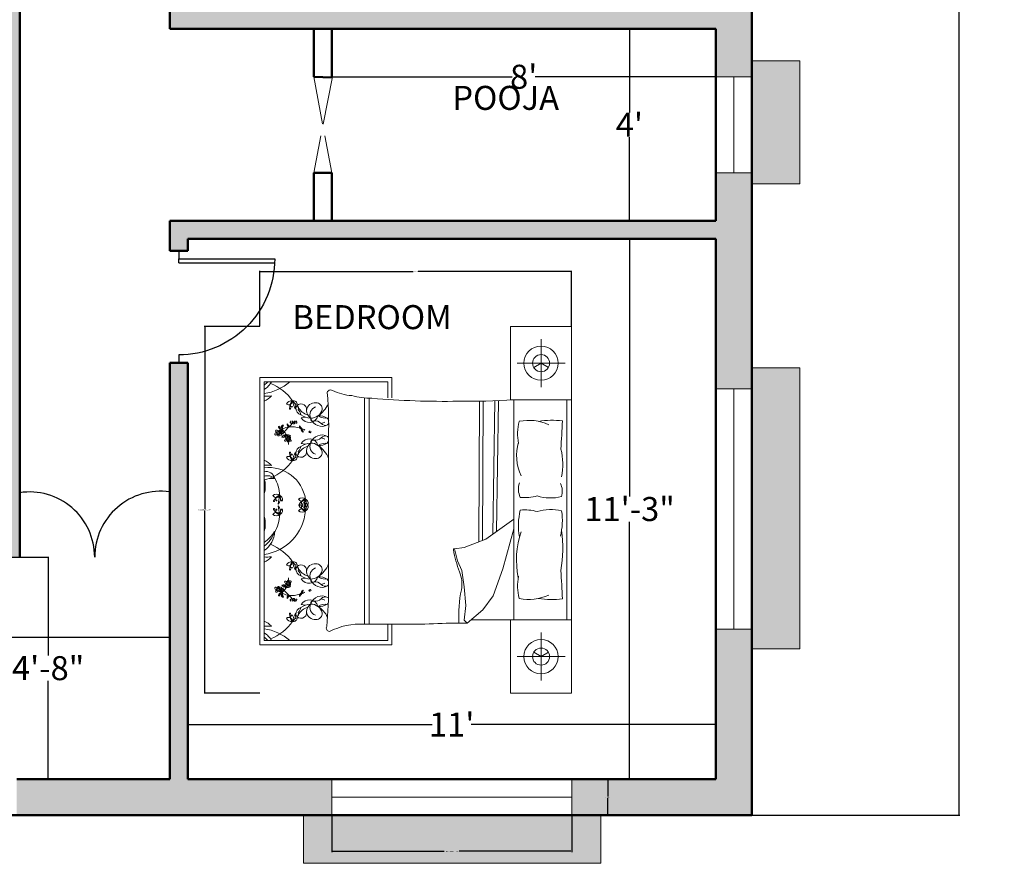
# Model space of a CAD drawing. Units: inches. Extents: x -28 to 544, y -640 to 52.
# Tile 3 of 11: x 297 to 544, y -600 to -389. Entities that reach past the tile are written whole.
import ezdxf

# ---------------------------------------------------------------- set-up
doc = ezdxf.new("R2010")
doc.units = ezdxf.units.IN
doc.header["$MEASUREMENT"] = 0
doc.linetypes.add('ACAD_ISO02W100', pattern=[15, 12, -3])
for name, color, linetype, lineweight in [('A-ANNO-DIMS', 2, 'Continuous', 18), ('A-AREA-IDEN', 7, 'Continuous', 25), ('A-DOOR', 3, 'Continuous', 25), ('A-FLOR-STRS', 7, 'Continuous', 25), ('A-FURN', 8, 'Continuous', 18), ('A-GLAZ', 4, 'Continuous', 20), ('A-ROOF', 8, 'Continuous', 18), ('A-ROOF-PATT', 252, 'Continuous', 13), ('A-WALL', 7, 'Continuous', 50), ('A-WALL-OVHD', 8, 'ACAD_ISO02W100', 18), ('A-WALL-PATT', 5, 'Continuous', 13)]:
    doc.layers.add(name, color=color, linetype=linetype, lineweight=lineweight)
doc.styles.get("Standard").update_dxf_attribs({"font": 'arial.ttf'})
doc.dimstyles.get("Standard").update_dxf_attribs({"dimtxt": 0.18, "dimasz": 0.18, "dimexe": 0.18, "dimexo": 0.0625, "dimgap": 0.09, "dimtad": 0, "dimtih": 1, "dimtoh": 1, "dimdec": 0, "dimzin": 0, "dimdsep": 46, "dimlunit": 3, "dimtxsty": 'Standard', "dimcen": 0.09, "dimadec": 0, "dimazin": 0, "dimtfac": 1, "dimtdec": 0, "dimtofl": 0, "dimtmove": 0, "dimatfit": 3, "dimfxl": 1, "dimtolj": 1, "dimtzin": 0, "dimarcsym": 0})

# ---------------------------------------------------------------- blocks, each defined once
blk = doc.blocks.new('*D23')
at = {"layer": 'A-ANNO-DIMS', "color": 0, "lineweight": -2, "transparency": 16777216}
for p, q in [((339.44, -566.16), (339.44, -564.9)), ((339.62, -565.08), (400.55, -565.08)), ((471.26, -565.08), (410.34, -565.08)), ((471.44, -566.16), (471.44, -564.9))]:
    blk.add_line(p, q, dxfattribs=at)
at = {"layer": 'A-ANNO-DIMS', "color": 0, "transparency": 16777216}
for points in [[(339.62, -565.05), (339.62, -565.11), (339.44, -565.08)], [(471.26, -565.05), (471.26, -565.11), (471.44, -565.08)]]:
    blk.add_solid(points, dxfattribs=at)
at = {"layer": 'Defpoints', "color": 0, "transparency": 16777216}
for p in [(471.44, -565.08), (339.44, -566.22), (471.44, -566.22)]:
    blk.add_point(p, dxfattribs=at)
at = {"layer": 'A-ANNO-DIMS', "color": 0, "transparency": 16777216, "insert": (405.44, -565.08), "char_height": 6, "attachment_point": 5}
blk.add_mtext("\\A1;11'", dxfattribs=at)
blk = doc.blocks.new('*D24')
at = {"layer": 'A-ANNO-DIMS', "color": 0, "lineweight": -2, "transparency": 16777216}
for p, q in [((449.91, -443.92), (449.91, -508.09)), ((449.97, -443.74), (450.09, -443.74)), ((449.91, -578.56), (449.91, -514.4)), ((449.97, -578.74), (450.09, -578.74))]:
    blk.add_line(p, q, dxfattribs=at)
at = {"layer": 'A-ANNO-DIMS', "color": 0, "transparency": 16777216}
for points in [[(449.88, -443.92), (449.94, -443.92), (449.91, -443.74)], [(449.88, -578.56), (449.94, -578.56), (449.91, -578.74)]]:
    blk.add_solid(points, dxfattribs=at)
at = {"layer": 'Defpoints', "color": 0, "transparency": 16777216}
for p in [(449.91, -443.74), (449.91, -578.74), (449.91, -578.74)]:
    blk.add_point(p, dxfattribs=at)
at = {"layer": 'A-ANNO-DIMS', "color": 0, "transparency": 16777216, "insert": (449.91, -511.24), "char_height": 6, "attachment_point": 5}
blk.add_mtext('\\A1;11\'-3"', dxfattribs=at)
blk = doc.blocks.new('*D28')
at = {"layer": 'A-ANNO-DIMS', "color": 0, "lineweight": -2, "transparency": 16777216}
for p, q in [((480.51, 7.76), (532.47, 7.76)), ((532.29, 7.58), (532.29, -286.84)), ((532.29, -587.56), (532.29, -293.14)), ((480.51, -587.74), (532.47, -587.74))]:
    blk.add_line(p, q, dxfattribs=at)
at = {"layer": 'A-ANNO-DIMS', "color": 0, "transparency": 16777216}
for points in [[(532.26, 7.58), (532.32, 7.58), (532.29, 7.76)], [(532.26, -587.56), (532.32, -587.56), (532.29, -587.74)]]:
    blk.add_solid(points, dxfattribs=at)
at = {"layer": 'Defpoints', "color": 0, "transparency": 16777216}
for p in [(480.44, 7.76), (480.44, -587.74), (532.29, -587.74)]:
    blk.add_point(p, dxfattribs=at)
at = {"layer": 'A-ANNO-DIMS', "color": 0, "transparency": 16777216, "insert": (532.29, -289.99), "char_height": 6, "attachment_point": 5}
blk.add_mtext('\\A1;49\'-8"', dxfattribs=at)
blk = doc.blocks.new('*D31')
at = {"layer": 'A-ANNO-DIMS', "color": 0, "lineweight": -2, "transparency": 16777216}
for p, q in [((375.44, -397.6), (375.44, -403.42)), ((471.44, -397.6), (471.44, -403.42)), ((375.62, -403.24), (420.59, -403.24)), ((471.26, -403.24), (426.3, -403.24))]:
    blk.add_line(p, q, dxfattribs=at)
at = {"layer": 'A-ANNO-DIMS', "color": 0, "transparency": 16777216}
for points in [[(375.62, -403.21), (375.62, -403.27), (375.44, -403.24)], [(471.26, -403.21), (471.26, -403.27), (471.44, -403.24)]]:
    blk.add_solid(points, dxfattribs=at)
at = {"layer": 'Defpoints', "color": 0, "transparency": 16777216}
for p in [(375.44, -397.54), (471.44, -397.54), (471.44, -403.24)]:
    blk.add_point(p, dxfattribs=at)
at = {"layer": 'A-ANNO-DIMS', "color": 0, "transparency": 16777216, "insert": (423.44, -403.24), "char_height": 6, "attachment_point": 5}
blk.add_mtext("\\A1;8'", dxfattribs=at)
blk = doc.blocks.new('*D32')
at = {"layer": 'A-ANNO-DIMS', "color": 0, "lineweight": -2, "transparency": 16777216}
for p, q in [((453.92, -391.24), (449.68, -391.24)), ((449.86, -391.42), (449.86, -412.15)), ((449.86, -439.06), (449.86, -418.33)), ((453.92, -439.24), (449.68, -439.24))]:
    blk.add_line(p, q, dxfattribs=at)
at = {"layer": 'A-ANNO-DIMS', "color": 0, "transparency": 16777216}
for points in [[(449.83, -391.42), (449.89, -391.42), (449.86, -391.24)], [(449.83, -439.06), (449.89, -439.06), (449.86, -439.24)]]:
    blk.add_solid(points, dxfattribs=at)
at = {"layer": 'Defpoints', "color": 0, "transparency": 16777216}
for p in [(453.98, -391.24), (449.86, -439.24), (453.98, -439.24)]:
    blk.add_point(p, dxfattribs=at)
at = {"layer": 'A-ANNO-DIMS', "color": 0, "transparency": 16777216, "insert": (449.86, -415.24), "char_height": 6, "attachment_point": 5}
blk.add_mtext("\\A1;4'", dxfattribs=at)
blk = doc.blocks.new('*D41')
at = {"layer": 'A-ANNO-DIMS', "color": 0, "lineweight": -2, "transparency": 16777216}
for p, q in [((162.44, -543.27), (162.44, -543.15)), ((162.62, -543.33), (238.58, -543.33)), ((334.76, -543.33), (258.81, -543.33)), ((334.94, -543.27), (334.94, -543.15))]:
    blk.add_line(p, q, dxfattribs=at)
at = {"layer": 'A-ANNO-DIMS', "color": 0, "transparency": 16777216}
for points in [[(162.62, -543.3), (162.62, -543.36), (162.44, -543.33)], [(334.76, -543.3), (334.76, -543.36), (334.94, -543.33)]]:
    blk.add_solid(points, dxfattribs=at)
at = {"layer": 'Defpoints', "color": 0, "transparency": 16777216}
for p in [(162.44, -543.33), (334.94, -543.33), (334.94, -543.33)]:
    blk.add_point(p, dxfattribs=at)
at = {"layer": 'A-ANNO-DIMS', "color": 0, "transparency": 16777216, "insert": (248.69, -543.33), "char_height": 6, "attachment_point": 5}
blk.add_mtext('\\A1;14\'-5"', dxfattribs=at)
blk = doc.blocks.new('*D42')
at = {"layer": 'A-ANNO-DIMS', "color": 0, "lineweight": -2, "transparency": 16777216}
for p, q in [((297.51, -523.24), (304.73, -523.24)), ((304.55, -523.42), (304.55, -547.84)), ((304.55, -578.56), (304.55, -554.14)), ((301.15, -578.74), (304.73, -578.74))]:
    blk.add_line(p, q, dxfattribs=at)
at = {"layer": 'A-ANNO-DIMS', "color": 0, "transparency": 16777216}
for points in [[(304.52, -523.42), (304.58, -523.42), (304.55, -523.24)], [(304.52, -578.56), (304.58, -578.56), (304.55, -578.74)]]:
    blk.add_solid(points, dxfattribs=at)
at = {"layer": 'Defpoints', "color": 0, "transparency": 16777216}
for p in [(297.44, -523.24), (301.09, -578.74), (304.55, -578.74)]:
    blk.add_point(p, dxfattribs=at)
at = {"layer": 'A-ANNO-DIMS', "color": 0, "transparency": 16777216, "insert": (304.55, -550.99), "char_height": 6, "attachment_point": 5}
blk.add_mtext('\\A1;4\'-8"', dxfattribs=at)
blk = doc.blocks.new('BED-DOUBLE-HEADBOARD-92')
for p, q in [((77.93, 0), (77.93, 91.63)), ((70.29, 76.48), (70.29, 88.45)), ((64.3, 82.47), (76.28, 82.47)), ((0, 78.9), (0, 12.09)), ((33.01, 78.9), (0, 78.9)), ((33.01, 73.82), (33.01, 78.9)), ((1.06, 77.84), (31.95, 77.84)), ((1.06, 13.16), (1.06, 77.84)), ((31.95, 77.84), (31.95, 73.8)), ((26.15, 73.81), (26.15, 17.27)), ((27.29, 73.72), (27.29, 17.27)), ((54.87, 72.98), (54.73, 37.82)), ((55.81, 72.98), (55.68, 38.18)), ((58.7, 73.02), (58.23, 39.75)), ((59.64, 73.06), (59.18, 40.44)), ((63.45, 18.33), (63.45, 73.3)), ((76.75, 73.3), (76.75, 18.33)), ((10.35, 68.81), (11.39, 69.01)), ((17.15, 64.42), (17.15, 27.21)), ((10.35, 62.4), (11.39, 62.2)), ((63.45, 43.5), (56.46, 38.48)), ((60.72, 31.05), (63.45, 41.05)), ((56.46, 38.48), (51.08, 36.44)), ((51.08, 36.44), (48.67, 36.07)), ((48.67, 36.07), (49.41, 33.1)), ((49.41, 33.1), (50.52, 30.68)), ((50.52, 30.68), (51.08, 26.6)), ((58.31, 24.37), (60.72, 31.05)), ((10.35, 28.59), (11.39, 28.79)), ((51.08, 26.6), (51.45, 21.96)), ((10.35, 22.19), (11.39, 21.98)), ((55.71, 20.85), (58.31, 24.37)), ((51.45, 21.96), (51.08, 18.25)), ((51.82, 17.51), (55.71, 20.85)), ((31.95, 17.28), (31.95, 13.16)), ((33.01, 12.09), (33.01, 17.28)), ((51.08, 18.25), (51.82, 17.51)), ((77.93, 18.33), (52.78, 18.33)), ((70.29, 15.15), (70.29, 3.18)), ((31.95, 13.16), (1.06, 13.16)), ((0, 12.09), (33.01, 12.09)), ((64.3, 9.16), (76.28, 9.16))]:
    blk.add_line(p, q)
for points in [[(77.93, 73.3), (62.65, 73.3), (62.65, 91.63), (77.93, 91.63)], [(70.29, 82.47), (68.44, 81.4)], [(70.29, 82.47), (72.14, 81.4)], [(62.65, 18.33), (62.65, 0), (77.93, 0)], [(70.29, 9.16), (68.44, 10.23)], [(70.29, 9.16), (72.14, 10.23)]]:
    blk.add_lwpolyline(points)
for points in [[(28.01, 73.7, -0.056112), (22.97, 74.36, -0.095341), (18.12, 75.65)], [(75.64, 68.04, 0.074897), (69.66, 67.93, -0.472817)], [(69.32, 49.3, 0.14099), (75.43, 49.12, 0.235245)], [(69.32, 45.39, -0.14099), (75.43, 45.57, -0.235245)], [(75.64, 23.59, -0.074897), (69.66, 23.7, 0.472817)], [(43.43, 17.31, -0.001242), (26.04, 17.27, 0.127202), (17.38, 15.43)]]:
    blk.add_lwpolyline(points, format="xyb")
for centre, radius in [((70.29, 82.47), 4.28), ((70.29, 82.47), 2.14), ((4.57, 65.04), 0.233), ((7.03, 63.51), 0.233), ((7.03, 27.48), 0.233), ((4.57, 25.95), 0.233), ((70.29, 9.16), 4.28), ((70.29, 9.16), 2.14)]:
    blk.add_circle(centre, radius)
for centre, radius, start, end in [((-2.15, 80.74), 5.83, 303.4617, 330.1116), ((-3.24, 82.84), 7.27, 306.3036, 316.4814), ((-0.55, 86.74), 11.97, 277.745, 311.8856), ((-1.73, 66.27), 11.97, 34.3865, 68.5908), ((-0.8, 77.48), 4.87, 292.5547, 318.9546), ((1.81, 90.8), 16.56, 267.4081, 273.6519), ((17.65, 74.95), 0.835, 56.1736, 203.4781), ((-71.97, 67.22), 89.16, 358.1965, 4.7598), ((7.86, 71.73), 1.33, 77.7115, 159.0387), ((7.14, 73.06), 0.999, 238.4633, 358.2869), ((10.42, 71.04), 3.03, 138.8402, 177.9352), ((8.6, 72.16), 0.979, 117.6827, 223.7762), ((8.03, 71.59), 0.078, 223.7729, 159.7333), ((8.38, 72.07), 0.992, 2.9516, 103.728), ((16.31, 74.84), 8.37, 192.5173, 207.1824), ((7.04, 71.5), 1.89, 345.4653, 54.2343), ((9.89, 74.09), 2.04, 211.3827, 255.2969), ((10.28, 70.9), 1.38, 350.264, 160.8688), ((8.79, 71.18), 0.843, 333.9755, 53.2681), ((13.81, 70.4), 2.19, 84.9449, 172.8857), ((14.64, 69.54), 2.13, 111.5819, 201.4221), ((14.03, 71.03), 1.55, 354.4856, 91.0538), ((10.7, 75.07), 6.94, 303.6671, 336.3547), ((46.26, 287.69), 214.77, 265.1265, 270.8855), ((52.25, 237.57), 164.64, 269.0718, 273.9), ((7.54, 71.14), 0.149, 177.9352, 11.4834), ((7.62, 71.16), 0.0722, 11.4834, 127.9409), ((10.69, 71.23), 1.72, 175.969, 254.3045), ((8.41, 69.38), 1.83, 6.1662, 51.5825), ((13.3, 73.63), 4.33, 211.2614, 251.7045), ((12.96, 73.67), 4.92, 236.2883, 266.5076), ((12.33, 69.94), 2.28, 209.9085, 343.1337), ((14.29, 70.78), 2.66, 182.3591, 234.0401), ((12.88, 71.51), 2.76, 265.2933, 346.921), ((16.47, 72.53), 3.8, 238.8218, 280.751), ((14.82, 65.78), 3.53, 55.785, 94.7304), ((4.91, 66.54), 0.261, 124.3538, 214.3923), ((5.47, 66.72), 0.705, 176.9701, 248.2913), ((10.5, 70.44), 6.82, 212.6784, 216.3746), ((5.88, 66.37), 0.608, 122.8155, 187.3992), ((6.14, 66.29), 0.705, 109.4799, 177.6828), ((5.76, 66.74), 0.261, 56.8636, 146.9021), ((5.9, 66.45), 0.27, 148.8844, 224.2646), ((11.5, 63.06), 6.82, 145.1882, 148.8844), ((7.62, 62.77), 3.8, 94.756, 119.2041), ((15.72, 57.29), 12.52, 132.2412, 142.1744), ((9.4, 67.26), 2.58, 178.3264, 187.1302), ((6.61, 66.9), 0.481, 11.3256, 64.4621), ((8.24, 67.59), 1.45, 190.2588, 210.656), ((7.27, 67), 0.44, 188.3432, 274.2869), ((7.66, 67.24), 0.768, 210.656, 242.6341), ((8.24, 67.9), 1.47, 218.2101, 226.3071), ((7.15, 66.67), 0.187, 325.7657, 67.4417), ((1.35, 72.91), 8.7, 313.1541, 322.0459), ((7.81, 58.99), 7.59, 73.5842, 93.8277), ((7.75, 67.68), 0.179, 142.4737, 265.053), ((7.99, 67.72), 0.385, 127.7621, 169.0403), ((7.78, 68.04), 0.542, 265.053, 338.3618), ((8.5, 67.3), 0.709, 113.4276, 137.6104), ((8.42, 68.04), 0.233, 183.2768, 356.7232), ((8.59, 67.61), 0.382, 139.7889, 227.6792), ((8.47, 67.48), 0.201, 227.6792, 350.3487), ((7.69, 67.62), 0.764, 353.0852, 15.7171), ((8.19, 67.53), 0.482, 350.3487, 43.6538), ((9.08, 68.03), 0.561, 198.7263, 262.5032), ((8.64, 67.76), 0.223, 1.1081, 91.8675), ((9.06, 67.64), 0.18, 255.2356, 54.9248), ((8.78, 67.71), 0.389, 11.5637, 52.6358), ((12.48, 66.71), 2.58, 178.3264, 187.1302), ((9.69, 66.35), 0.481, 11.3256, 64.4621), ((11.32, 67.04), 1.45, 190.2588, 210.656), ((13.28, 68.5), 0.569, 167.3041, 285.1471), ((14.82, 65.78), 3.53, 122.7011, 126.3445), ((15.49, 69.59), 2.92, 199.2822, 299.1751), ((13.92, 66.14), 1.88, 41.5653, 105.1471), ((14.96, 70.03), 2.63, 277.436, 299.9149), ((16.35, 68.29), 1.37, 221.5653, 293.8354), ((16.14, 67.83), 1.1, 17.4186, 52.325), ((16.14, 67.83), 1.1, 314.4517, 343.3657), ((76.71, 64.77), 12.28, 165.1039, 191.0369), ((67.25, 56.37), 11.81, 65.1316, 101.7583), ((947.66, 17.54), 873.48, 176.68521, 177.14978), ((3.9, 64.68), 0.179, 142.4737, 265.053), ((4.14, 64.72), 0.385, 61.2196, 169.0403), ((3.93, 65.05), 0.542, 265.053, 338.3618), ((4.39, 65.51), 0.461, 157.4086, 261.4386), ((4.13, 65.53), 0.231, 58.0499, 135.6268), ((4.65, 64.3), 0.709, 113.4276, 137.6104), ((4.37, 65.38), 0.155, 172.906, 277.132), ((3.87, 65.1), 0.736, 14.7558, 58.0499), ((4.74, 64.62), 0.382, 139.7889, 227.6792), ((4.62, 64.48), 0.201, 227.6792, 350.3487), ((4.9, 65.3), 0.318, 36.1046, 181.4281), ((3.84, 64.62), 0.764, 353.0852, 15.7171), ((4.34, 64.53), 0.482, 350.3487, 43.6538), ((5.29, 66.5), 0.608, 190.3057, 287.1958), ((4.71, 65.55), 0.321, 270.0645, 331.1507), ((4.98, 65.47), 0.367, 221.8413, 265.7877), ((5.24, 65.03), 0.561, 198.7263, 262.5032), ((4.79, 64.77), 0.223, 1.1081, 91.8675), ((4.98, 65.33), 0.229, 263.7526, 41.7054), ((4.93, 64.72), 0.389, 11.5637, 86.365), ((5.23, 66.56), 0.27, 216.3746, 291.7548), ((7.62, 62.77), 3.8, 124.0033, 132.4917), ((5.21, 64.65), 0.18, 255.2356, 54.9248), ((3.7, 62.29), 4.06, 63.7819, 68.2913), ((5.88, 65.42), 0.647, 128.3208, 208.8162), ((5.99, 65.47), 0.773, 207.7043, 254.3516), ((5.41, 66.12), 0.204, 289.3605, 111.7548), ((5.56, 66.12), 0.204, 221.8703, 44.2646), ((6.48, 65.52), 1.06, 157.2305, 229.0635), ((5.49, 65.02), 1.06, 270.278, 342.111), ((6.2, 63.69), 0.752, 98.7227, 159.3375), ((6.12, 65.88), 0.626, 174.4544, 220.6188), ((2.56, 62.38), 4.56, 30.544, 49.818), ((5.08, 64.98), 0.752, 340.0041, 40.6188), ((5.99, 65.06), 0.626, 278.7227, 324.8872), ((5.88, 64.55), 0.647, 290.5253, 358.5375), ((6.85, 63.99), 0.461, 157.4086, 261.4386), ((6.59, 64), 0.231, 58.0499, 135.6268), ((7.14, 64.73), 0.647, 182.8499, 266.1226), ((6.89, 65.19), 0.626, 231.7607, 277.9252), ((7.38, 65.3), 1.06, 214.5369, 286.3699), ((6.33, 63.57), 0.736, 14.7558, 58.0499), ((2.56, 62.38), 4.56, 23.0501, 23.8477), ((7.08, 63.82), 0.752, 37.3105, 97.9252), ((7.36, 63.77), 0.318, 36.1046, 181.4281), ((7.16, 64.86), 0.773, 265.0106, 311.658), ((10.35, 66.45), 0.44, 188.3432, 274.2869), ((10.74, 66.7), 0.768, 210.656, 242.6341), ((11.32, 67.36), 1.47, 218.2101, 226.3071), ((10.23, 66.12), 0.187, 325.7657, 67.4417), ((10.76, 65.78), 0.44, 147.5332, 233.4768), ((11.15, 66), 0.768, 179.1859, 211.164), ((10.41, 65.83), 0.187, 354.3784, 96.0543), ((7.81, 58.99), 7.59, 63.0032, 69.8941), ((11.99, 67.54), 2.58, 234.6898, 243.4936), ((11.74, 66.36), 1.45, 211.164, 231.5612), ((12.01, 66.21), 1.47, 195.5129, 203.6099), ((10.35, 65.24), 0.481, 357.3579, 50.4944), ((12.42, 65.34), 0.177, 12.7051, 190.4384), ((12.53, 65.36), 0.287, 190.4384, 10.4136), ((15.49, 61.62), 2.92, 60.8249, 160.7178), ((16.35, 62.91), 1.37, 66.1646, 138.4347), ((16.14, 63.38), 1.1, 23.2856, 45.5483), ((5.82, 64.66), 0.773, 244.9899, 291.6373), ((6.36, 63.16), 0.179, 142.4737, 265.053), ((6.6, 63.19), 0.385, 61.2196, 169.0403), ((6.39, 63.52), 0.542, 265.053, 338.3618), ((7.11, 62.78), 0.709, 113.4276, 137.6104), ((6.83, 63.86), 0.155, 172.906, 277.132), ((7.2, 63.09), 0.382, 139.7889, 227.6792), ((7.08, 62.96), 0.201, 227.6792, 350.3487), ((6.3, 63.09), 0.764, 353.0852, 15.7171), ((2.56, 62.38), 4.56, 357.1071, 4.7585), ((6.8, 63), 0.482, 350.3487, 43.6538), ((7.17, 64.02), 0.321, 270.0645, 331.1507), ((7.44, 63.94), 0.367, 221.8413, 265.7877), ((7.7, 63.5), 0.561, 198.7263, 262.5032), ((7.25, 63.24), 0.223, 1.1081, 91.8675), ((7.44, 63.81), 0.229, 263.7526, 41.7054), ((7.39, 63.19), 0.389, 11.5637, 86.365), ((7.67, 63.12), 0.18, 255.2356, 54.9248), ((10.69, 59.98), 1.72, 105.6955, 184.031), ((8.41, 61.83), 1.83, 308.4175, 353.8338), ((13.3, 57.58), 4.33, 108.2955, 148.7386), ((12.96, 57.54), 4.92, 93.4924, 123.7117), ((12.33, 61.27), 2.28, 16.8663, 150.0915), ((14.29, 60.43), 2.66, 125.9599, 177.6409), ((14.64, 61.67), 2.13, 158.5779, 248.4181), ((12.88, 59.7), 2.76, 13.079, 94.7067), ((13.28, 62.71), 0.569, 74.8529, 192.6959), ((14.82, 65.43), 3.53, 233.6555, 237.2989), ((13.92, 65.07), 1.88, 254.8529, 318.4347), ((16.47, 58.68), 3.8, 79.7133, 121.1782), ((14.82, 65.43), 3.53, 265.2696, 304.215), ((10.7, 56.14), 6.94, 21.4941, 56.3329), ((14.96, 61.18), 2.63, 60.0851, 82.564), ((16.14, 63.38), 1.1, 307.675, 336.7144), ((75.81, 59.47), 11.66, 163.8254, 206.1239), ((7.14, 58.15), 0.999, 1.7131, 121.5367), ((7.54, 60.07), 0.149, 348.5166, 182.0648), ((10.42, 60.17), 3.03, 182.0648, 221.1598), ((7.62, 60.05), 0.0722, 232.0591, 348.5166), ((8.6, 59.04), 0.979, 136.2238, 242.3173), ((7.98, 59.63), 0.129, 200.2817, 136.2238), ((7.04, 59.71), 1.89, 305.7657, 14.5347), ((16.31, 56.36), 8.37, 152.8176, 167.4827), ((8.38, 59.14), 0.992, 256.272, 357.0484), ((9.89, 57.11), 2.04, 104.7031, 148.6173), ((10.28, 60.31), 1.38, 199.1312, 9.736), ((8.79, 60.02), 0.843, 306.7319, 26.0245), ((13.81, 60.81), 2.19, 187.1143, 275.0551), ((14.03, 60.18), 1.55, 268.9462, 5.5144), ((59.61, 57.17), 16.11, 348.8159, 13.6573), ((-0.8, 53.73), 4.87, 41.0454, 67.4453), ((1.81, 40.41), 16.56, 86.3481, 92.5919), ((-1.73, 64.94), 11.97, 291.4092, 325.6135), ((7.86, 59.47), 1.33, 200.9613, 282.2885), ((2.21, 47.13), 9.26, 8.1803, 97.1364), ((1.57, 53.24), 2.15, 10.9261, 103.6102), ((1.86, 51.63), 2.72, 48.0951, 107.1391), ((-5.23, 51.78), 6.58, 343.5431, 17.0202), ((3.06, 48.33), 5.36, 83.3805, 111.883), ((-6.96, 48.43), 11.97, 4.4623, 27.4146), ((69.49, 50.99), 4.86, 161.4593, 204.9817), ((71.07, 50.37), 4.53, 343.8974, 26.6563), ((-8.62, 49.17), 9.73, 4.3787, 5.6357), ((-15.29, 44.05), 17.39, 19.7217, 19.9028), ((4.08, 48.38), 1.33, 47.7873, 129.1145), ((4.12, 49.89), 0.999, 208.5391, 328.3627), ((5.95, 46.5), 3.03, 108.9159, 148.011), ((4.93, 48.39), 0.979, 87.7585, 193.852), ((12.96, 46.86), 8.37, 162.593, 177.2582), ((3.25, 48.59), 1.89, 315.5411, 24.3101), ((7.01, 49.42), 2.04, 181.4585, 225.3727), ((4.69, 48.41), 0.992, 333.0274, 73.8037), ((66.26, 60.1), 11.23, 264.0129, 285.8293), ((3.51, 48.03), 0.149, 148.011, 341.5592), ((3.58, 48), 0.0722, 341.5592, 98.0167), ((4.16, 48.17), 0.078, 193.9791, 129.8091), ((12.96, 47.19), 8.37, 182.7418, 197.407), ((3.25, 45.46), 1.89, 335.6899, 44.4589), ((10.49, 47.47), 1.33, 47.7873, 129.1145), ((10.53, 48.97), 0.999, 208.5391, 328.3627), ((9.92, 47.11), 0.149, 148.011, 341.5592), ((9.92, 46.94), 0.149, 18.4408, 211.989), ((12.36, 45.59), 3.03, 108.9159, 148.011), ((12.36, 48.46), 3.03, 211.989, 251.0841), ((9.99, 47.09), 0.0722, 341.5592, 98.0167), ((9.99, 46.96), 0.0722, 261.9833, 18.4408), ((11.34, 47.47), 0.979, 87.7585, 193.852), ((11.34, 46.58), 0.979, 166.148, 272.2415), ((10.52, 46.78), 0.129, 230.0755, 166.148), ((10.57, 47.26), 0.078, 193.9791, 129.8091), ((9.65, 47.67), 1.89, 315.5411, 24.3101), ((19.37, 45.95), 8.37, 162.593, 177.2582), ((9.65, 46.38), 1.89, 335.6899, 44.4589), ((19.37, 48.1), 8.37, 182.7418, 197.407), ((11.1, 47.5), 0.992, 333.0274, 73.8037), ((13.42, 48.5), 2.04, 181.4585, 225.3727), ((11.1, 46.55), 0.992, 286.1963, 26.9726), ((13.42, 45.55), 2.04, 134.6273, 178.5415), ((-0.55, 46.53), 11.97, 277.745, 355.5377), ((4.12, 44.16), 0.999, 31.6373, 151.4609), ((4.08, 45.66), 1.33, 230.8855, 312.2127), ((3.51, 46.02), 0.149, 18.4408, 211.989), ((5.95, 47.54), 3.03, 211.989, 251.0841), ((3.58, 46.04), 0.0722, 261.9833, 18.4408), ((-6.96, 45.61), 11.97, 332.5854, 355.5377), ((4.93, 45.66), 0.979, 166.148, 272.2415), ((4.11, 45.86), 0.129, 230.0755, 166.148), ((7.01, 44.63), 2.04, 134.6273, 178.5415), ((4.69, 45.63), 0.992, 286.1963, 26.9726), ((10.53, 45.07), 0.999, 31.6373, 151.4609), ((10.49, 46.58), 1.33, 230.8855, 312.2127), ((80.79, 41.94), 16.16, 166.3762, 190.1383), ((66.26, 34.58), 11.23, 74.1707, 95.9871), ((59.28, 43.16), 16.33, 346.04, 8.4751), ((-5.23, 42.27), 6.58, 342.9798, 16.4569), ((-8.62, 44.87), 9.73, 354.3643, 355.6213), ((-15.29, 50), 17.39, 340.0972, 340.2783), ((-2.15, 40.53), 5.83, 303.4617, 358.728), ((-5.28, 46.44), 10.81, 305.947, 325.9877), ((-3.24, 42.62), 7.27, 306.3036, 342.1496), ((85.44, 33.32), 21.3, 160.7385, 191.9603), ((42.48, 36.14), 33.23, 350.503, 7.7804), ((-1.73, 26.06), 11.97, 34.3865, 68.5908), ((48.59, 35.86), 0.221, 70.2464, 181.1377), ((83.29, 42.43), 35.54, 190.6617, 199.8806), ((1.81, 50.59), 16.56, 267.4081, 273.6519), ((-0.8, 37.26), 4.87, 292.5547, 318.9546), ((7.86, 31.52), 1.33, 77.7115, 159.0387), ((7.14, 32.84), 0.999, 238.4633, 358.2869), ((10.42, 30.82), 3.03, 138.8402, 177.9352), ((8.6, 31.95), 0.979, 117.6827, 223.7762), ((8.38, 31.85), 0.992, 2.9516, 103.728), ((9.89, 33.88), 2.04, 211.3827, 255.2969), ((7.04, 31.28), 1.89, 345.4653, 54.2343), ((16.31, 34.63), 8.37, 192.5173, 207.1824), ((10.28, 30.69), 1.38, 350.264, 160.8688), ((13.81, 30.18), 2.19, 84.9449, 172.8857), ((14.03, 30.82), 1.55, 354.4856, 91.0538), ((10.7, 34.86), 6.94, 303.6671, 338.5059), ((7.54, 30.93), 0.149, 177.9352, 11.4834), ((7.62, 30.94), 0.0722, 11.4834, 127.9409), ((8.03, 31.37), 0.078, 223.7729, 159.7333), ((10.69, 31.02), 1.72, 175.969, 254.3045), ((8.79, 30.97), 0.843, 333.9755, 53.2681), ((8.41, 29.17), 1.83, 6.1662, 51.5825), ((13.3, 33.41), 4.33, 211.2614, 251.7045), ((14.29, 30.56), 2.66, 182.3591, 234.0401), ((14.64, 29.32), 2.13, 111.5819, 201.4221), ((12.88, 31.29), 2.76, 265.2933, 346.921), ((43.05, 27.34), 7.46, 348.6608, 23.7384), ((947.66, 74.1), 873.48, 182.85022, 183.31479), ((5.82, 26.33), 0.773, 68.3627, 115.0101), ((6.36, 27.83), 0.179, 94.947, 217.5263), ((6.6, 27.8), 0.385, 190.9597, 298.7804), ((6.39, 27.47), 0.542, 21.6382, 94.947), ((6.85, 27), 0.461, 98.5614, 202.5914), ((7.11, 28.21), 0.709, 222.3896, 246.5724), ((6.83, 27.13), 0.155, 82.868, 187.094), ((6.33, 27.42), 0.736, 301.9501, 345.2442), ((7.2, 27.9), 0.382, 132.3208, 220.2111), ((7.08, 28.04), 0.201, 9.6513, 132.3208), ((6.3, 27.9), 0.764, 344.2829, 6.9148), ((7.36, 27.22), 0.318, 178.5719, 323.8954), ((2.56, 28.61), 4.56, 355.2415, 2.8929), ((6.8, 27.99), 0.482, 316.3462, 9.6513), ((7.7, 27.49), 0.561, 97.4968, 161.2737), ((7.44, 27.05), 0.367, 94.2123, 138.1587), ((7.17, 26.97), 0.321, 28.8493, 89.9355), ((7.25, 27.75), 0.223, 268.1325, 358.8919), ((7.39, 27.8), 0.389, 273.635, 348.4363), ((7.44, 27.19), 0.229, 318.2946, 96.2474), ((7.67, 27.87), 0.18, 305.0752, 104.7644), ((12.96, 33.45), 4.92, 236.2883, 266.5076), ((12.33, 29.73), 2.28, 209.9085, 343.1337), ((13.28, 28.28), 0.569, 167.3041, 285.1471), ((14.82, 25.56), 3.53, 122.7011, 126.3445), ((15.49, 29.37), 2.92, 199.2822, 299.1751), ((13.92, 25.92), 1.88, 41.5653, 105.1471), ((16.47, 32.31), 3.8, 238.8218, 280.2867), ((14.82, 25.56), 3.53, 55.785, 94.7304), ((14.96, 29.81), 2.63, 277.436, 299.9149), ((16.35, 28.08), 1.37, 221.5653, 293.8354), ((-78.23, 26.12), 95.39, 354.3113, 0.6567), ((16.14, 27.61), 1.1, 23.2856, 52.325), ((16.14, 27.61), 1.1, 314.4517, 336.771), ((76.71, 26.86), 12.28, 168.9631, 194.8961), ((3.9, 26.31), 0.179, 94.947, 217.5263), ((4.14, 26.27), 0.385, 190.9597, 298.7804), ((3.93, 25.95), 0.542, 21.6382, 94.947), ((4.39, 25.48), 0.461, 98.5614, 202.5914), ((4.13, 25.46), 0.231, 224.3732, 301.9501), ((4.65, 26.69), 0.709, 222.3896, 246.5724), ((4.37, 25.61), 0.155, 82.868, 187.094), ((3.87, 25.89), 0.736, 301.9501, 345.2442), ((4.74, 26.38), 0.382, 132.3208, 220.2111), ((4.62, 26.51), 0.201, 9.6513, 132.3208), ((3.84, 26.37), 0.764, 344.2829, 6.9148), ((4.9, 25.7), 0.318, 178.5719, 323.8954), ((4.34, 26.46), 0.482, 316.3462, 9.6513), ((5.29, 24.49), 0.608, 72.8042, 169.6943), ((5.24, 25.96), 0.561, 97.4968, 161.2737), ((4.98, 25.52), 0.367, 94.2123, 138.1587), ((4.71, 25.45), 0.321, 28.8493, 89.9355), ((5.47, 24.27), 0.705, 111.7087, 183.0299), ((4.79, 26.23), 0.223, 268.1325, 358.8919), ((4.93, 26.28), 0.389, 273.635, 348.4363), ((4.98, 25.66), 0.229, 318.2946, 96.2474), ((5.23, 24.44), 0.27, 68.2452, 143.6254), ((7.62, 28.22), 3.8, 227.5083, 235.9967), ((5.21, 26.35), 0.18, 305.0752, 104.7644), ((3.7, 28.7), 4.06, 291.7087, 296.2181), ((5.88, 25.57), 0.647, 151.1838, 231.6792), ((5.88, 24.62), 0.608, 172.6008, 237.1845), ((5.99, 25.53), 0.773, 105.6484, 152.2957), ((5.41, 24.88), 0.204, 248.2452, 70.6395), ((5.56, 24.88), 0.204, 315.7354, 138.1297), ((6.48, 25.47), 1.06, 130.9365, 202.7695), ((6.14, 24.7), 0.705, 182.3172, 250.5201), ((5.49, 25.97), 1.06, 17.889, 89.722), ((6.2, 27.3), 0.752, 200.6625, 261.2773), ((6.12, 25.12), 0.626, 139.3812, 185.5456), ((2.56, 28.61), 4.56, 310.182, 329.456), ((5.9, 24.55), 0.27, 135.7354, 211.1156), ((5.08, 26.01), 0.752, 319.3812, 19.9959), ((7.62, 28.22), 3.8, 240.7959, 265.244), ((15.72, 33.7), 12.52, 217.8256, 227.7588), ((5.99, 25.94), 0.626, 35.1128, 81.2773), ((5.88, 26.45), 0.647, 1.4625, 69.4747), ((6.59, 26.99), 0.231, 224.3732, 301.9501), ((7.14, 26.26), 0.647, 93.8774, 177.1501), ((7.38, 25.69), 1.06, 73.6301, 145.4631), ((6.89, 25.81), 0.626, 82.0748, 128.2393), ((2.56, 28.61), 4.56, 336.1523, 336.9499), ((7.08, 27.17), 0.752, 262.0748, 322.6895), ((7.16, 26.14), 0.773, 48.342, 94.9894), ((7.81, 32), 7.59, 266.1723, 286.4158), ((11.32, 23.95), 1.45, 149.344, 169.7412), ((10.35, 24.54), 0.44, 85.7131, 171.6568), ((10.74, 24.29), 0.768, 117.3659, 149.344), ((11.32, 23.63), 1.47, 133.6929, 141.7899), ((10.23, 24.87), 0.187, 292.5583, 34.2343), ((10.76, 25.21), 0.44, 126.5232, 212.4668), ((11.15, 24.99), 0.768, 148.836, 180.8141), ((10.41, 25.16), 0.187, 263.9457, 5.6216), ((7.81, 32), 7.59, 290.1059, 296.9968), ((11.99, 23.46), 2.58, 116.5064, 125.3102), ((11.74, 24.64), 1.45, 128.4388, 148.836), ((12.01, 24.79), 1.47, 156.3901, 164.4871), ((10.35, 25.75), 0.481, 309.5056, 2.6421), ((12.42, 25.65), 0.177, 169.5616, 347.2949), ((12.53, 25.63), 0.287, 349.5864, 169.5616), ((84.27, 19.07), 34.58, 168.6608, 182.5481), ((4.91, 24.45), 0.261, 145.6077, 235.6462), ((10.5, 20.55), 6.82, 143.6254, 147.3216), ((5.76, 24.26), 0.261, 213.0979, 303.1364), ((11.5, 27.93), 6.82, 211.1156, 214.8118), ((9.4, 23.73), 2.58, 172.8698, 181.6736), ((8.24, 23.4), 1.45, 149.344, 169.7412), ((6.61, 24.09), 0.481, 295.5379, 348.6744), ((7.27, 23.99), 0.44, 85.7131, 171.6568), ((7.66, 23.75), 0.768, 117.3659, 149.344), ((8.24, 23.09), 1.47, 133.6929, 141.7899), ((7.15, 24.33), 0.187, 292.5583, 34.2343), ((1.35, 18.08), 8.7, 37.9541, 46.8459), ((7.75, 23.31), 0.179, 94.947, 217.5263), ((7.99, 23.27), 0.385, 190.9597, 232.2379), ((7.78, 22.95), 0.542, 21.6382, 94.947), ((8.5, 23.69), 0.709, 222.3896, 246.5724), ((8.42, 22.96), 0.233, 3.2768, 176.7232), ((8.59, 23.38), 0.382, 132.3208, 220.2111), ((8.47, 23.51), 0.201, 9.6513, 132.3208), ((7.69, 23.37), 0.764, 344.2829, 6.9148), ((8.19, 23.46), 0.482, 316.3462, 9.6513), ((9.08, 22.97), 0.561, 97.4968, 161.2737), ((8.64, 23.23), 0.223, 268.1325, 358.8919), ((9.06, 23.35), 0.18, 305.0752, 104.7644), ((8.78, 23.28), 0.389, 307.3642, 348.4363), ((12.48, 24.28), 2.58, 172.8698, 181.6736), ((9.69, 24.64), 0.481, 295.5379, 348.6744), ((12.96, 17.32), 4.92, 93.4924, 123.7117), ((12.33, 21.05), 2.28, 16.8663, 150.0915), ((14.29, 20.21), 2.66, 125.9599, 177.6409), ((14.64, 21.45), 2.13, 158.5779, 248.4181), ((12.88, 19.48), 2.76, 13.079, 94.7067), ((13.28, 22.49), 0.569, 74.8529, 192.6959), ((15.49, 21.4), 2.92, 60.8249, 160.7178), ((14.82, 25.21), 3.53, 233.6555, 237.2989), ((13.92, 24.86), 1.88, 254.8529, 318.4347), ((16.47, 18.46), 3.8, 80.8446, 121.1782), ((14.82, 25.21), 3.53, 265.2696, 304.215), ((14.96, 20.96), 2.63, 60.0851, 82.564), ((16.35, 22.7), 1.37, 66.1646, 138.4347), ((16.14, 23.17), 1.1, 307.675, 329.9707), ((16.14, 23.17), 1.1, 26.442, 45.5483), ((67.25, 35.26), 11.81, 258.2417, 294.8684), ((7.54, 19.85), 0.149, 348.5166, 182.0648), ((10.42, 19.95), 3.03, 182.0648, 221.1598), ((7.62, 19.83), 0.0722, 232.0591, 348.5166), ((16.31, 16.15), 8.37, 152.8176, 167.4827), ((7.04, 19.5), 1.89, 305.7657, 14.5347), ((10.69, 19.76), 1.72, 105.6955, 184.031), ((10.28, 20.09), 1.38, 199.1312, 9.736), ((8.79, 19.81), 0.843, 306.7319, 26.0245), ((8.41, 21.61), 1.83, 308.4175, 353.8338), ((13.3, 17.36), 4.33, 108.2955, 148.7386), ((13.81, 20.59), 2.19, 187.1143, 275.0551), ((14.03, 19.96), 1.55, 268.9462, 5.5144), ((10.7, 15.92), 6.94, 26.7003, 56.3329), ((-0.8, 13.52), 4.87, 41.0454, 67.4453), ((-1.73, 24.72), 11.97, 291.4092, 325.6135), ((7.14, 17.93), 0.999, 1.7131, 121.5367), ((7.86, 19.26), 1.33, 200.9613, 282.2885), ((8.6, 18.83), 0.979, 136.2238, 242.3173), ((7.98, 19.42), 0.129, 200.2817, 136.2238), ((9.89, 16.9), 2.04, 104.7031, 148.6173), ((8.38, 18.93), 0.992, 256.272, 357.0484), ((49.54, -66.51), 84.05, 88.447, 94.1706), ((1.81, 0.19), 16.56, 86.3481, 92.5919), ((-0.55, 4.25), 11.97, 48.1144, 82.255), ((-2.15, 10.25), 5.83, 29.8884, 56.5383), ((17.44, 16.28), 0.845, 152.6588, 266.02), ((-3.24, 8.15), 7.27, 43.5186, 53.6964)]:
    blk.add_arc(centre, radius, start, end)
blk = doc.blocks.new('WIN-60IN')
for p, q in [((0, 9), (60, 9)), ((0, 0), (0, 9)), ((60, 9), (60, 0)), ((0, 4.5), (60, 4.5)), ((60, 0), (0, 0))]:
    blk.add_line(p, q)
blk = doc.blocks.new('WIN-24IN')
for p, q in [((0, 0), (0, 24)), ((0, 24), (9, 24)), ((4.5, 0), (4.5, 24)), ((9, 24), (9, 0)), ((9, 0), (0, 0))]:
    blk.add_line(p, q)
blk = doc.blocks.new('DOOR-SWING-24IN')
for p, q in [((25, 0), (25, 24)), ((26, 0), (26, 24)), ((2, 0), (0, 0)), ((25, 0), (26, 0)), ((28, 0), (26, 0))]:
    blk.add_line(p, q)
blk.add_arc((26, 0), 24, 90, 180)
blk = doc.blocks.new('*D57')
at = {"layer": 'A-ANNO-DIMS', "color": 0, "lineweight": -2, "transparency": 16777216}
for p, q in [((375.44, -587.8), (375.44, -596.92)), ((435.44, -587.8), (435.44, -596.92)), ((375.62, -596.74), (403.54, -596.74)), ((435.26, -596.74), (407.35, -596.74))]:
    blk.add_line(p, q, dxfattribs=at)
at = {"layer": 'A-ANNO-DIMS', "color": 0, "transparency": 16777216}
for points in [[(375.62, -596.71), (375.62, -596.77), (375.44, -596.74)], [(435.26, -596.71), (435.26, -596.77), (435.44, -596.74)]]:
    blk.add_solid(points, dxfattribs=at)
at = {"layer": 'Defpoints', "color": 0, "transparency": 16777216}
for p in [(375.44, -587.74), (435.44, -587.74), (435.44, -596.74)]:
    blk.add_point(p, dxfattribs=at)
at = {"layer": 'A-ANNO-DIMS', "color": 0, "transparency": 16777216, "insert": (405.44, -596.74), "char_height": 0.18, "attachment_point": 5}
blk.add_mtext('\\A1;BEDROOM WINDOW 5\'-0" TYP.', dxfattribs=at)
blk = doc.blocks.new('*D58')
at = {"layer": 'A-ANNO-DIMS', "color": 0, "lineweight": -2, "transparency": 16777216}
for p, q in [((435.51, -578.74), (444.62, -578.74)), ((444.44, -578.92), (444.44, -583.06)), ((444.44, -587.56), (444.44, -583.42)), ((435.51, -587.74), (444.62, -587.74))]:
    blk.add_line(p, q, dxfattribs=at)
at = {"layer": 'A-ANNO-DIMS', "color": 0, "transparency": 16777216}
for points in [[(444.41, -578.92), (444.47, -578.92), (444.44, -578.74)], [(444.41, -587.56), (444.47, -587.56), (444.44, -587.74)]]:
    blk.add_solid(points, dxfattribs=at)
at = {"layer": 'Defpoints', "color": 0, "transparency": 16777216}
for p in [(435.44, -578.74), (444.44, -578.74), (435.44, -587.74)]:
    blk.add_point(p, dxfattribs=at)
at = {"layer": 'A-ANNO-DIMS', "color": 0, "transparency": 16777216, "insert": (444.44, -583.24), "char_height": 0.18, "attachment_point": 5}
blk.add_mtext('\\A1;0\'-9" TYP.', dxfattribs=at)
blk = doc.blocks.new('*D69')
at = {"layer": 'A-ANNO-DIMS', "color": 0, "lineweight": -2, "transparency": 16777216}
for p, q in [((357.44, -465.63), (343.58, -465.63)), ((343.76, -465.81), (343.76, -511.26)), ((343.76, -557.08), (343.76, -511.63)), ((357.44, -557.26), (343.58, -557.26))]:
    blk.add_line(p, q, dxfattribs=at)
at = {"layer": 'A-ANNO-DIMS', "color": 0, "transparency": 16777216}
for points in [[(343.73, -465.81), (343.79, -465.81), (343.76, -465.63)], [(343.73, -557.08), (343.79, -557.08), (343.76, -557.26)]]:
    blk.add_solid(points, dxfattribs=at)
at = {"layer": 'Defpoints', "color": 0, "transparency": 16777216}
for p in [(343.76, -465.63), (357.5, -465.63), (357.5, -557.26)]:
    blk.add_point(p, dxfattribs=at)
at = {"layer": 'A-ANNO-DIMS', "color": 0, "transparency": 16777216, "insert": (343.76, -511.44), "char_height": 0.18, "attachment_point": 5}
blk.add_mtext('\\A1;DOUBLE BED C 7\'-7 1/2" TYP.', dxfattribs=at)
blk = doc.blocks.new('*D70')
at = {"layer": 'A-ANNO-DIMS', "color": 0, "lineweight": -2, "transparency": 16777216}
for p, q in [((357.5, -465.57), (357.5, -451.7)), ((357.68, -451.88), (395.82, -451.88)), ((435.25, -451.88), (397.1, -451.88)), ((435.43, -465.57), (435.43, -451.7))]:
    blk.add_line(p, q, dxfattribs=at)
at = {"layer": 'A-ANNO-DIMS', "color": 0, "transparency": 16777216}
for points in [[(357.68, -451.85), (357.68, -451.91), (357.5, -451.88)], [(435.25, -451.85), (435.25, -451.91), (435.43, -451.88)]]:
    blk.add_solid(points, dxfattribs=at)
at = {"layer": 'Defpoints', "color": 0, "transparency": 16777216}
for p in [(435.43, -451.88), (357.5, -465.63), (435.43, -465.63)]:
    blk.add_point(p, dxfattribs=at)
at = {"layer": 'A-ANNO-DIMS', "color": 0, "transparency": 16777216, "insert": (396.46, -451.88), "char_height": 0.18, "attachment_point": 5}
blk.add_mtext('\\A1;6\'-6" TYP.', dxfattribs=at)

msp = doc.modelspace()

# ---------------------------------------------------------------- hatches: boundary and pattern name
at = {"layer": 'A-ROOF-PATT'}
h = msp.add_hatch(color=256, dxfattribs=at)
h.dxf.hatch_style = 1
h.set_gradient(color1=(241, 235, 31), color2=(248, 153, 30))
h.paths.add_polyline_path([(124.53, 19.76), (58.75, 19.76), (58.75, 7.76), (124.53, 7.76)])
h.paths.add_polyline_path([(226.33, 19.76), (182.83, 19.76), (182.83, 7.76), (226.33, 7.76)])
h.paths.add_polyline_path([(313.67, 19.76), (271.84, 19.76), (271.84, 7.76), (313.67, 7.76)])
h.paths.add_polyline_path([(440.55, 19.76), (372.16, 19.76), (372.16, 7.76), (440.55, 7.76)])
h.paths.add_polyline_path([(492.44, -34.91), (480.44, -34.91), (480.44, -100.18), (492.44, -100.18)])
h.paths.add_polyline_path([(492.44, -151.37), (480.44, -151.37), (480.44, -179.02), (492.44, -179.02)])
h.paths.add_polyline_path([(492.44, -207.96), (480.44, -207.96), (480.44, -238.77), (492.44, -238.77)])
h.paths.add_polyline_path([(492.44, -289.99), (480.44, -289.99), (480.44, -354.53), (492.44, -354.53)])
h.paths.add_polyline_path([(492.44, -399.27), (480.44, -399.27), (480.44, -430), (492.44, -430)])
h.paths.add_polyline_path([(492.44, -475.99), (480.44, -475.99), (480.44, -546.14), (492.44, -546.14)])
h.paths.add_polyline_path([(442.7, -587.74), (368.43, -587.74), (368.43, -599.74), (442.7, -599.74)])
h.paths.add_polyline_path([(127.64, -587.74), (54.75, -587.74), (54.75, -599.74), (127.64, -599.74)])
h.paths.add_polyline_path([(16.94, -477.43), (4.94, -477.43), (4.94, -547.54), (16.94, -547.54)])
h.paths.add_polyline_path([(16.94, -399.8), (4.94, -399.8), (4.94, -430.58), (16.94, -430.58)])
h.paths.add_polyline_path([(16.94, -287.93), (4.94, -287.93), (4.94, -356.82), (16.94, -356.82)])
h.paths.add_polyline_path([(16.94, -208.93), (4.94, -208.93), (4.94, -240.18), (16.94, -240.18)])
h.paths.add_polyline_path([(16.94, -150), (4.94, -150), (4.94, -180.17), (16.94, -180.17)])
h.paths.add_polyline_path([(16.94, -32.89), (4.94, -32.89), (4.94, -101.73), (16.94, -101.73)])
at = {"layer": 'A-WALL-PATT'}
h = msp.add_hatch(color=256, dxfattribs=at)
h.dxf.hatch_style = 1
h.paths.add_polyline_path([(375.44, 7.76), (310.94, 7.76), (310.94, -1.24), (334.94, -1.24), (334.94, -133.24), (286.94, -133.24), (286.94, -137.74), (342.44, -137.74), (342.44, -133.24), (339.44, -133.24), (339.44, -1.24), (375.44, -1.24)])
h.paths.add_polyline_path([(480.44, 7.76), (435.44, 7.76), (435.44, -1.24), (471.44, -1.24), (471.44, -37.24), (480.44, -37.24)])
h.paths.add_polyline_path([(480.44, -97.24), (471.44, -97.24), (471.44, -133.24), (417.44, -133.24), (417.44, -135.49), (417.44, -137.74), (471.44, -137.74), (471.44, -152.74), (480.44, -152.74)])
h.paths.add_polyline_path([(480.44, -176.74), (471.44, -176.74), (471.44, -191.74), (387.44, -191.74), (387.44, -137.74), (389.44, -137.74), (389.44, -133.24), (370.44, -133.24), (370.44, -135.49), (370.44, -137.74), (382.94, -137.74), (382.94, -191.74), (382.94, -196.24), (382.94, -220.24), (385.19, -220.24), (387.44, -220.24), (387.44, -196.24), (471.44, -196.24), (471.44, -211.24), (480.44, -211.24)])
h.paths.add_polyline_path([(480.44, -235.24), (471.44, -235.24), (471.44, -250.24), (387.44, -250.24), (387.44, -248.24), (382.94, -248.24), (382.94, -250.24), (369.44, -250.24), (369.44, -252.49), (369.44, -254.74), (471.44, -254.74), (471.44, -290.74), (480.44, -290.74)])
h.paths.add_polyline_path([(480.44, -350.74), (471.44, -350.74), (471.44, -386.74), (339.44, -386.74), (339.44, -254.74), (341.44, -254.74), (341.44, -250.24), (334.94, -250.24), (334.94, -391.24), (471.44, -391.24), (471.44, -403.24), (480.44, -403.24)])
h.paths.add_polyline_path([(480.44, -427.24), (471.44, -427.24), (471.44, -439.24), (334.94, -439.24), (334.94, -446.74), (339.44, -446.74), (339.44, -443.74), (471.44, -443.74), (471.44, -481.24), (480.44, -481.24)])
h.paths.add_polyline_path([(480.44, -541.24), (471.44, -541.24), (471.44, -578.74), (435.44, -578.74), (435.44, -587.74), (480.44, -587.74)])
h.paths.add_polyline_path([(375.44, -578.74), (339.44, -578.74), (339.44, -474.74), (337.19, -474.74), (334.94, -474.74), (334.94, -578.74), (296.69, -578.74), (296.69, -587.74), (375.44, -587.74)])
h = msp.add_hatch(color=256, dxfattribs=at)
h.dxf.hatch_style = 1
h.paths.add_polyline_path([(246.44, -386.74), (199.94, -386.74), (199.94, -391.24), (199.94, -523.24), (205.44, -523.24), (205.44, -391.24), (246.44, -391.24), (246.44, -433.24), (250.94, -433.24), (250.94, -391.24), (291.94, -391.24), (291.94, -523.24), (297.44, -523.24), (297.44, -386.74), (250.94, -386.74), (250.94, -250.24), (246.44, -250.24)])
h.paths.add_polyline_path([(244.06, -411.97), (253.32, -411.97), (253.32, -399.6), (244.06, -399.6)], flags=25)

# ---------------------------------------------------------------- linework, layer by layer
at = {"layer": 'A-DOOR'}
for centre, radius, start, end in [((299.93, -523.24), 16.26, 0, 98.8082), ((332.64, -523.24), 16.44, 81.9332, 180)]:
    msp.add_arc(centre, radius, start, end, dxfattribs=at)
at = {"layer": 'A-FLOR-STRS'}
msp.add_line((291.94, -523.24), (297.44, -523.24), dxfattribs=at)
at = {"layer": 'A-ROOF'}
for p, q in [((480.44, -399.27), (492.44, -399.27)), ((492.44, -399.27), (492.44, -430)), ((492.44, -430), (480.44, -430)), ((480.44, -475.99), (492.44, -475.99)), ((492.44, -475.99), (492.44, -546.14)), ((492.44, -546.14), (480.44, -546.14)), ((368.43, -587.74), (368.43, -599.74)), ((442.7, -599.74), (442.7, -587.74)), ((368.43, -599.74), (442.7, -599.74))]:
    msp.add_line(p, q, dxfattribs=at)
at = {"layer": 'A-WALL'}
for p, q in [((480.44, 7.76), (480.44, -587.74)), ((334.94, -250.24), (334.94, -391.24)), ((297.44, -523.24), (297.44, -386.74)), ((334.94, -391.24), (471.44, -391.24)), ((370.94, -391.24), (370.94, -403.24)), ((375.44, -391.24), (375.44, -403.42)), ((471.44, -391.24), (471.44, -439.24)), ((370.94, -403.24), (375.44, -403.42)), ((375.44, -427.24), (370.94, -427.24)), ((370.94, -427.24), (370.94, -439.24)), ((375.44, -427.24), (375.44, -439.24)), ((334.94, -439.24), (471.44, -439.24)), ((334.94, -439.24), (334.94, -446.74)), ((339.44, -443.74), (471.44, -443.74)), ((339.44, -443.74), (339.44, -446.74)), ((471.44, -443.74), (471.44, -578.74)), ((339.44, -446.74), (334.94, -446.74)), ((337.19, -474.74), (334.94, -474.74)), ((334.94, -474.74), (334.94, -578.74)), ((337.19, -474.74), (339.44, -474.74)), ((339.44, -474.74), (339.44, -578.74)), ((296.69, -578.74), (334.94, -578.74)), ((339.44, -578.74), (471.44, -578.74)), ((16.94, -587.74), (480.44, -587.74))]:
    msp.add_line(p, q, dxfattribs=at)
at = {"layer": 'A-WALL-OVHD'}
for p, q in [((370.94, -403.24), (375.44, -427.24)), ((375.62, -403.27), (370.94, -427.24))]:
    msp.add_line(p, q, dxfattribs=at)

# ---------------------------------------------------------------- block references
at = {"layer": 'A-DOOR', "extrusion": (0, 0, -1), "zscale": -1, "rotation": 89.99999999999999}
msp.add_blockref('DOOR-SWING-24IN', (-337.19, -474.74), dxfattribs=at)
at = {"layer": 'A-FURN'}
msp.add_blockref('BED-DOUBLE-HEADBOARD-92', (357.5, -557.26), dxfattribs=at)
at = {"layer": 'A-GLAZ'}
for name, p in [('WIN-24IN', (471.44, -427.24)), ('WIN-60IN', (375.44, -587.74))]:
    msp.add_blockref(name, p, dxfattribs=at)
at = {"layer": 'A-GLAZ', "rotation": 90.00000000000003}
msp.add_blockref('WIN-60IN', (480.44, -541.24), dxfattribs=at)

# ---------------------------------------------------------------- texts
at = {"layer": 'A-AREA-IDEN', "char_height": 6, "attachment_point": 1}
for s, insert in [('POOJA', (405.61, -405.52)), ('BEDROOM', (365.63, -460.3))]:
    msp.add_mtext(s, dxfattribs=dict(at, insert=insert))

# ---------------------------------------------------------------- dimensions: what is measured, and where the dimension line sits
at = {"layer": 'A-ANNO-DIMS'}
for base, p1, p2, picture, middle in [((532.28608123, -587.74117838), (480.44473605, 7.75882162), (480.44473605, -587.74117838), '*D28', (532.28608123, -289.99117838)), ((449.86, -439.24), (453.98, -391.24), (453.98, -439.24), '*D32', (449.86, -415.24)), ((449.91, -578.74), (449.91, -443.74), (449.91, -578.74), '*D24', (449.91, -511.24)), ((304.55174986, -578.74117838), (297.44473605, -523.24117838), (301.09042073, -578.74117838), '*D42', (304.55174986, -550.99117838))]:
    dim = msp.add_linear_dim(base=base, p1=p1, p2=p2, angle=90, dimstyle='Standard', override={"dimtxt": 6, "dimclrd": 0, "dimclre": 0, "dimclrt": 0}, dxfattribs=at)
    dim.commit()
    dim.dimension.update_dxf_attribs({"geometry": picture, "text_midpoint": middle})
for base, p1, p2, picture, middle in [((471.44, -403.24), (375.44, -397.54), (471.44, -397.54), '*D31', (423.44, -403.24)), ((334.94473605, -543.33075676), (162.44473605, -543.33075676), (334.94473605, -543.33075676), '*D41', (248.69473605, -543.33075676)), ((471.44, -565.08), (339.44, -566.22), (471.44, -566.22), '*D23', (405.44, -565.08))]:
    dim = msp.add_linear_dim(base=base, p1=p1, p2=p2, dimstyle='Standard', override={"dimtxt": 6, "dimclrd": 0, "dimclre": 0, "dimclrt": 0}, dxfattribs=at)
    dim.commit()
    dim.dimension.update_dxf_attribs({"geometry": picture, "text_midpoint": middle})
for base, p1, p2, text, picture, middle in [((435.43, -451.88), (357.5, -465.63), (435.43, -465.63), '<> TYP.', '*D70', (396.46, -451.88)), ((435.44, -596.74), (375.44, -587.74), (435.44, -587.74), 'BEDROOM WINDOW <> TYP.', '*D57', (405.44, -596.74))]:
    dim = msp.add_linear_dim(base=base, p1=p1, p2=p2, text=text, dimstyle='Standard', override={"dimdec": 1, "dimlfac": 1, "dimrnd": 0, "dimzin": 1, "dimdsep": 46, "dimlunit": 4, "dimfrac": 2}, dxfattribs=at)
    dim.commit()
    dim.dimension.update_dxf_attribs({"geometry": picture, "text_midpoint": middle})
for base, p1, p2, text, picture, middle in [((343.76, -465.63), (357.5, -557.26), (357.5, -465.63), 'DOUBLE BED C <> TYP.', '*D69', (343.76, -511.44)), ((444.44, -578.74), (435.44, -587.74), (435.44, -578.74), '<> TYP.', '*D58', (444.44, -583.24))]:
    dim = msp.add_linear_dim(base=base, p1=p1, p2=p2, angle=90, text=text, dimstyle='Standard', override={"dimdec": 1, "dimlfac": 1, "dimrnd": 0, "dimzin": 1, "dimdsep": 46, "dimlunit": 4, "dimfrac": 2}, dxfattribs=at)
    dim.commit()
    dim.dimension.update_dxf_attribs({"geometry": picture, "text_midpoint": middle})

doc.saveas('drawing.dxf')
